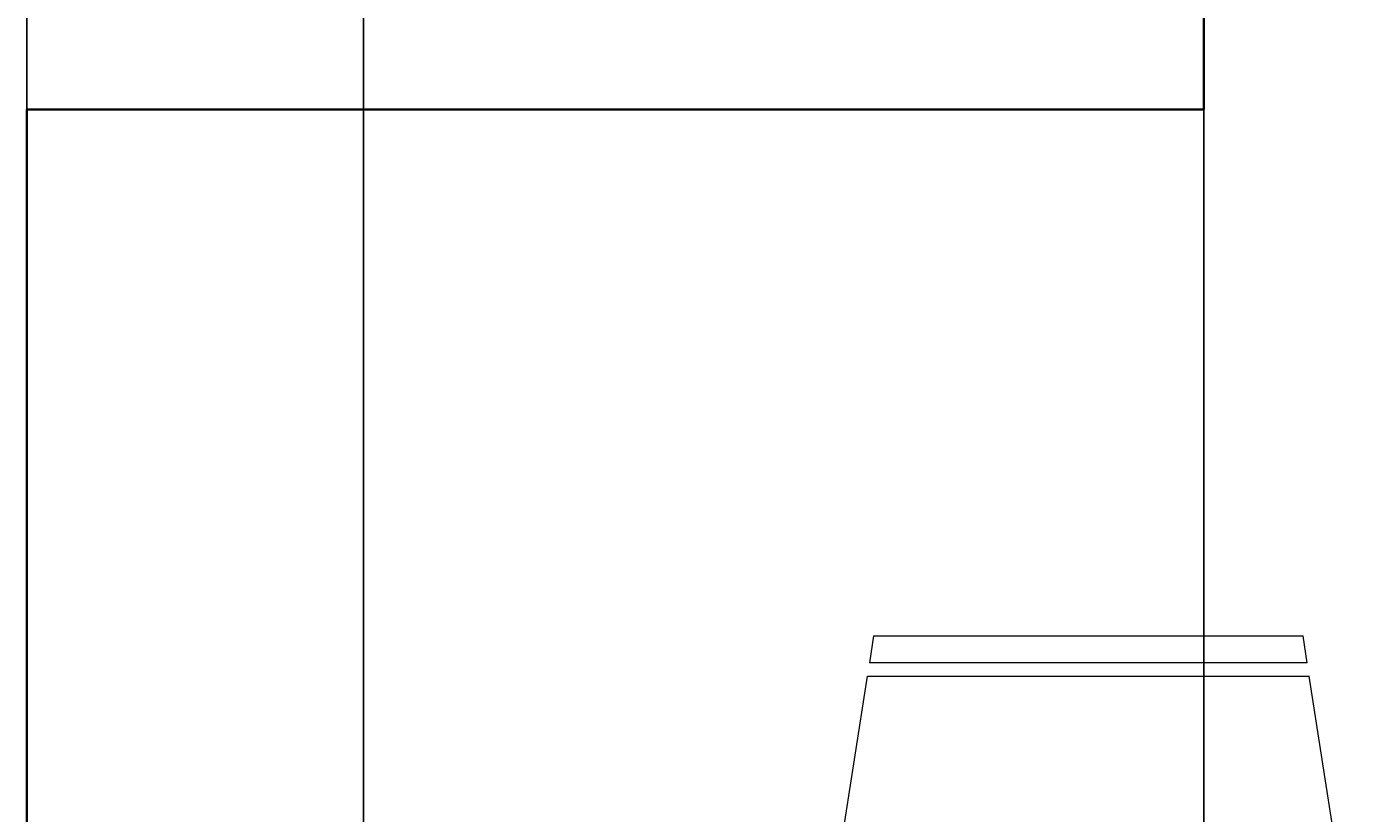
# Model space of a CAD drawing. Units: feet. Extents: x 1654 to 2985, y 1348 to 2230.
# Tile 30 of 53: x 1957 to 2002, y 1863 to 1889. Entities that reach past the tile are written whole.
import ezdxf

# ---------------------------------------------------------------- set-up
doc = ezdxf.new("R2010")
doc.units = ezdxf.units.FT
for name, color, linetype, lineweight in [('A-ANNO-DIMS', 2, 'Continuous', 18), ('A-FURN', 8, 'Continuous', 13), ('A-WALL', 7, 'Continuous', 35)]:
    doc.layers.add(name, color=color, linetype=linetype, lineweight=lineweight)
doc.styles.get("Standard").update_dxf_attribs({"font": 'arial.ttf'})
doc.dimstyles.get("Standard").update_dxf_attribs({"dimtxt": 0.18, "dimasz": 0.18, "dimexe": 0.18, "dimexo": 0.0625, "dimgap": 0.09, "dimtad": 0, "dimtih": 1, "dimtoh": 1, "dimdec": 4, "dimzin": 0, "dimdsep": 46, "dimtxsty": 'Standard', "dimcen": 0.09, "dimadec": 0, "dimazin": 0, "dimtfac": 1, "dimtdec": 4, "dimtofl": 0, "dimtmove": 0, "dimatfit": 3, "dimfxl": 1, "dimtolj": 1, "dimtzin": 0, "dimarcsym": 0})

# ---------------------------------------------------------------- blocks, each defined once
blk = doc.blocks.new('Dining Set - 36 x 72 in.')
for p, q in [((44.0006, 8.23428), (35.9976, 9.48474)), ((44, 8.23041), (44, -8.23915)), ((44.5, -8.15843), (44.5, 8.15338)), ((45.5, 8), (44.5005, 8.15617)), ((45.5, 8), (45.5, -8)), ((44.4997, -8.15631), (45.5, -8)), ((35.9976, -9.48476), (43.9993, -8.2345))]:
    blk.add_line(p, q)
blk = doc.blocks.new('*D97')
at = {"layer": 'A-ANNO-DIMS', "color": 0, "lineweight": -2, "transparency": 16777216}
for p, q in [((1957.092, 2108.192), (1957.092, 1534.075)), ((1968.254, 2108.192), (1968.254, 1534.075)), ((1957.272, 1534.255), (1962.219, 1534.255)), ((1968.074, 1534.255), (1963.128, 1534.255))]:
    blk.add_line(p, q, dxfattribs=at)
at = {"layer": 'A-ANNO-DIMS', "color": 0, "transparency": 16777216}
for points in [[(1957.272, 1534.285), (1957.272, 1534.225), (1957.092, 1534.255)], [(1968.074, 1534.285), (1968.074, 1534.225), (1968.254, 1534.255)]]:
    blk.add_solid(points, dxfattribs=at)
at = {"layer": 'Defpoints', "color": 0, "transparency": 16777216}
for p in [(1957.092, 2108.255), (1968.254, 2108.255), (1968.254, 1534.255)]:
    blk.add_point(p, dxfattribs=at)
at = {"layer": 'A-ANNO-DIMS', "color": 0, "transparency": 16777216, "insert": (1962.673, 1534.255), "char_height": 0.18, "attachment_point": 5}
blk.add_mtext('\\A1;11.162', dxfattribs=at)
blk = doc.blocks.new('*D101')
at = {"layer": 'A-ANNO-DIMS', "color": 0, "lineweight": -2, "transparency": 16777216}
for p, q in [((1996.092, 2039.192), (1996.092, 1534.075)), ((2014.016, 2039.192), (2014.016, 1534.075)), ((1996.272, 1534.255), (2004.599, 1534.255)), ((2013.836, 1534.255), (2005.509, 1534.255))]:
    blk.add_line(p, q, dxfattribs=at)
at = {"layer": 'A-ANNO-DIMS', "color": 0, "transparency": 16777216}
for points in [[(1996.272, 1534.285), (1996.272, 1534.225), (1996.092, 1534.255)], [(2013.836, 1534.285), (2013.836, 1534.225), (2014.016, 1534.255)]]:
    blk.add_solid(points, dxfattribs=at)
at = {"layer": 'Defpoints', "color": 0, "transparency": 16777216}
for p in [(1996.092, 2039.255), (2014.016, 2039.255), (2014.016, 1534.255)]:
    blk.add_point(p, dxfattribs=at)
at = {"layer": 'A-ANNO-DIMS', "color": 0, "transparency": 16777216, "insert": (2005.054, 1534.255), "char_height": 0.18, "attachment_point": 5}
blk.add_mtext('\\A1;17.924', dxfattribs=at)

msp = doc.modelspace()

# ---------------------------------------------------------------- linework, layer by layer
at = {"layer": 'A-WALL'}
for p, q in [((1996.0924, 1886.2549), (1996.0924, 1897.2549)), ((1957.0924, 1886.2549), (1996.0924, 1886.2549)), ((1957.0924, 1777.2549), (1957.0924, 1886.2549))]:
    msp.add_line(p, q, dxfattribs=at)

# ---------------------------------------------------------------- block references
at = {"layer": 'A-FURN', "xscale": 0.8893748792417884, "yscale": 0.8893748792417884, "zscale": 0.8893748792417884, "rotation": 90}
msp.add_blockref('Dining Set - 36 x 72 in.', (1992.2681, 1828.3522), dxfattribs=at)

# ---------------------------------------------------------------- dimensions: what is measured, and where the dimension line sits
at = {"layer": 'A-ANNO-DIMS'}
for base, p1, p2, picture, middle in [((1968.2542, 1534.2549), (1957.0924, 2108.2549), (1968.2542, 2108.2549), '*D97', (1962.6733, 1534.2549)), ((2014.016, 1534.2549), (1996.0924, 2039.2549), (2014.016, 2039.2549), '*D101', (2005.0542, 1534.2549))]:
    dim = msp.add_linear_dim(base=base, p1=p1, p2=p2, dimstyle='Standard', override={"dimdec": 3, "dimlfac": 1, "dimrnd": 0, "dimzin": 0, "dimdsep": 46, "dimlunit": 2}, dxfattribs=at)
    dim.commit()
    dim.dimension.update_dxf_attribs({"geometry": picture, "text_midpoint": middle})

doc.saveas('drawing.dxf')
